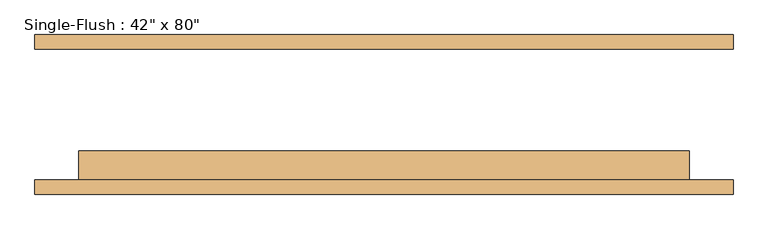
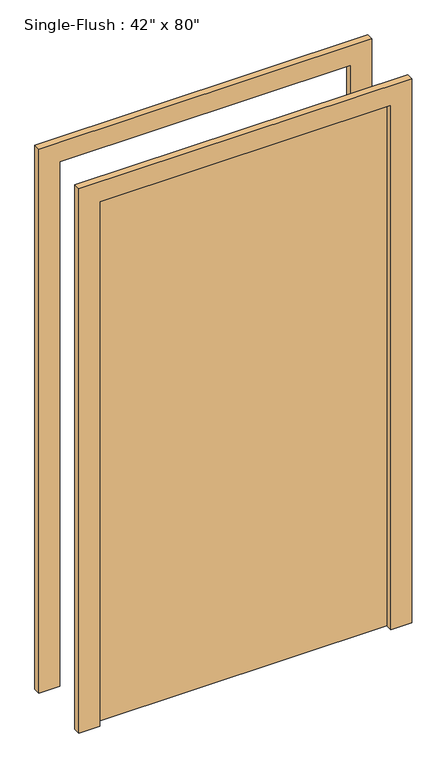
"""IFC4 building model written with IfcOpenShell, lengths in millimetres: door geometry."""

from ifc_helpers import new_model, si_unit, frame, origin, origin_with_axes, place, context, project, spatial, polyline, outline, extrude, source, transform, mapped, element, save


def door_f6232a3f(model_context):
    return source(origin(), model_context, "Body", "SweptSolid", [
        extrude(outline(polyline([(2108.2, -609.6), (0.0, -609.6), (0.0, -533.4), (2032.0, -533.4), (2032.0, 533.4), (0.0, 533.4), (0.0, 609.6), (2108.2, 609.6), (2108.2, -609.6)])), frame((0.0, -139.7, 0.0), z_axis=(0.0, 1.0, 0.0), x_axis=(0.0, 0.0, 1.0)), (0.0, 0.0, 1.0), 25.4),
        extrude(outline(polyline([(2108.2, 609.6), (2108.2, -609.6), (0.0, -609.6), (0.0, -533.4), (2032.0, -533.4), (2032.0, 533.4), (0.0, 533.4), (0.0, 609.6), (2108.2, 609.6)])), frame((0.0, 114.3, 0.0), z_axis=(0.0, 1.0, 0.0), x_axis=(0.0, 0.0, 1.0)), (0.0, 0.0, 1.0), 25.4),
        extrude(outline(polyline([(533.4, -63.5), (533.4, -114.3), (-533.4, -114.3), (-533.4, -63.5), (533.4, -63.5)])), origin_with_axes(), (0.0, 0.0, 1.0), 2032.0),
    ])


if __name__ == "__main__":
    model = new_model("IFC4")
    model_context = context("Model", 3, world=origin())
    ifc_project = project(units=[si_unit("LENGTHUNIT", "METRE", prefix="MILLI")], contexts=[model_context])
    site = spatial("IfcSite", under=ifc_project)
    building = spatial("IfcBuilding", under=site)
    placement = place(None, origin())
    door_shape = door_f6232a3f(model_context)
    element("IfcDoor", 1, ObjectType="Single-Flush : 42\" x 80\"", at=placement, inside=building, context=model_context, shape_type="MappedRepresentation", body=[
        mapped(door_shape, transform((0.0, 0.0, 0.0), x_axis=(1.0, 0.0, 0.0), y_axis=(0.0, 1.0, 0.0), z_axis=(0.0, 0.0, 1.0))),
    ])
    save(model, "model.ifc")

# Revit data of these elements
# Type "Single-Flush : 42\" x 80\""
#   Type Mark = "15"
#   Construction Type Id = "MDOOR"
#   Assembly Code = "C1020"
#   Analytic Construction = "Metal"
#   Thickness = 0' - 2"
#   Heat Transfer Coefficient (U) = 0.651978 BTU/(h·ft²·°F)
#   Height = 6' - 8"
#   Trim Projection Ext = 0' - 1"
#   Trim Projection Int = 0' - 1"
#   Trim Width = 0' - 3"
#   Width = 3' - 6"
#   Define Thermal Properties by = 1
#   Door Material = Door - Panel
#   Frame Material = Door - Frame
#   Visual Light Transmittance = 0
#   Solar Heat Gain Coefficient = 0
#   Function = (empty or 0)
#   Wall Closure = (empty or 0)
# Element 1 (IfcDoor, "Single-Flush : 42\" x 80\"")
#   Materials on its faces: "Door - Frame", "Door - Panel"
# Materials
#   "Door - Panel": class "Wood", colour RGB 210 159 95, transparency 0, Cost = 0
#   "Door - Frame": colour RGB 118 70 51, transparency 0, Cost = 0
